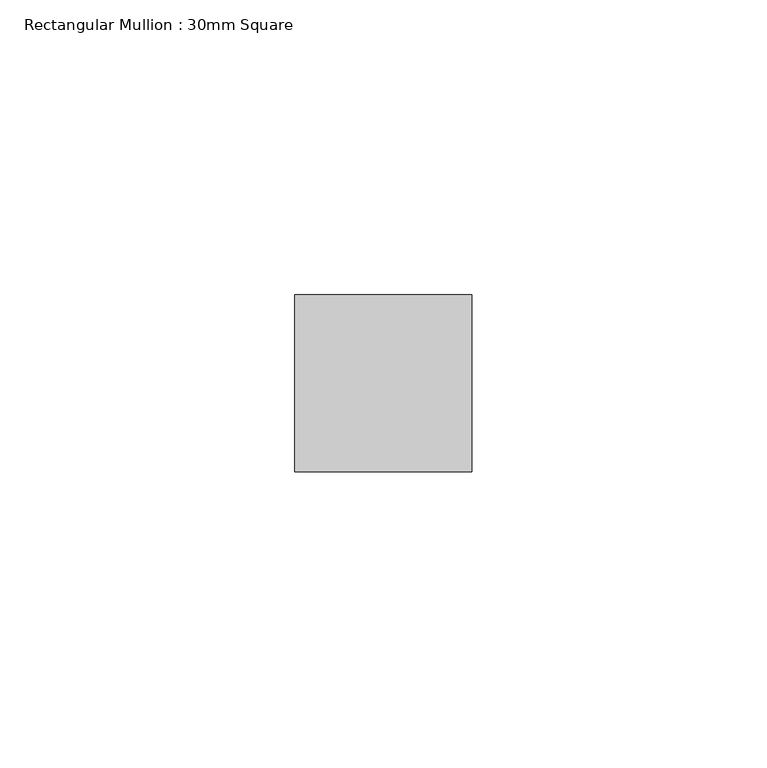
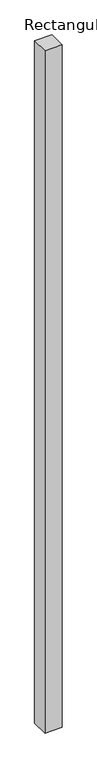
"""IFC4 building model written with IfcOpenShell, lengths in millimetres: member geometry, Rectangular Mullion : 30mm Square."""

from ifc_helpers import new_model, si_unit, frame, origin, place, context, project, spatial, polyline, outline, extrude, source, transform, mapped, element, save


def rectangular_mullion_30mm_square_e6372653(model_context):
    return source(origin(), model_context, "Body", "SweptSolid", [
        extrude(outline(polyline([(0.0, 15.0), (0.0, -15.0), (-30.0, -15.0), (-30.0, 15.0), (0.0, 15.0)])), frame((0.0, 0.0, -1237.5), z_axis=(0.0, 0.0, 1.0), x_axis=(1.0, 0.0, 0.0)), (0.0, 0.0, 1.0), 1237.5),
    ])


if __name__ == "__main__":
    model = new_model("IFC4")
    model_context = context("Model", 3, world=origin())
    ifc_project = project(units=[si_unit("LENGTHUNIT", "METRE", prefix="MILLI")], contexts=[model_context])
    site = spatial("IfcSite", under=ifc_project)
    building = spatial("IfcBuilding", under=site)
    placement = place(None, origin())
    rectangular_mullion_30mm_square_shape = rectangular_mullion_30mm_square_e6372653(model_context)
    element("IfcMember", 1, ObjectType="Rectangular Mullion : 30mm Square", at=placement, inside=building, context=model_context, shape_type="MappedRepresentation", body=[
        mapped(rectangular_mullion_30mm_square_shape, transform((0.0, 0.0, 0.0), x_axis=(1.0, 0.0, 0.0), y_axis=(0.0, 1.0, 0.0), z_axis=(0.0, 0.0, 1.0))),
    ])
    save(model, "model.ifc")

# Revit data of these elements
# Type "Rectangular Mullion : 30mm Square"
#   built-in parameter 1007304 = 0.0984252 (stored number, unit not read)
#   built-in parameter 1007301 = 0.0492126 (stored number, unit not read)
#   built-in parameter 1007300 = 0.0492126 (stored number, unit not read)
# Element 1 (IfcMember, "Rectangular Mullion : 30mm Square")
#   Materials on its faces: "Aluminum"
# Materials
#   "Aluminum": class "Metal", colour RGB 244 244 244, transparency 0, Description = "Aluminum 6061", Cost = 0
